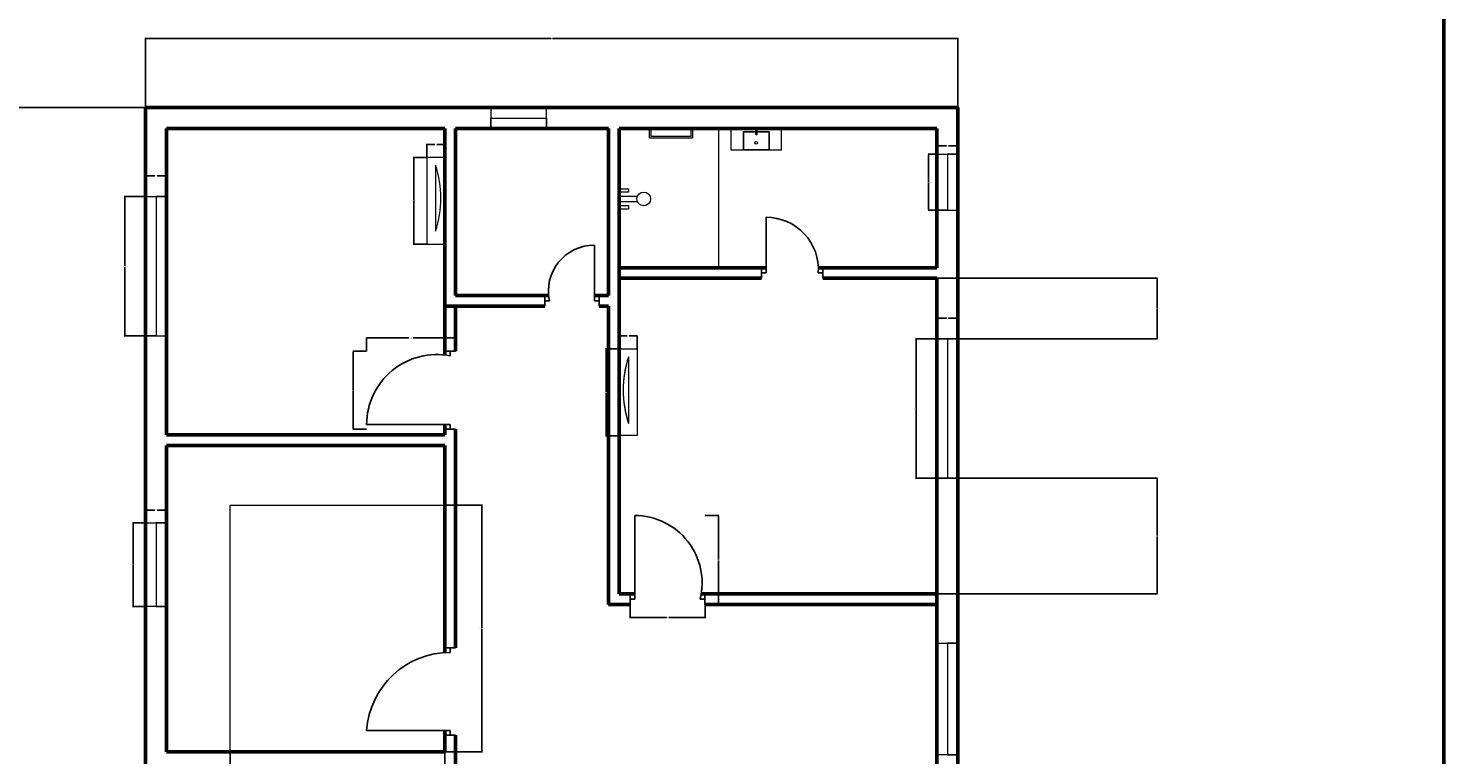
# Model space of a CAD drawing. Units: inches. Extents: x 2268 to 3372, y 1709 to 2892.
# Tile 5 of 6: x 2762 to 3372, y 2184 to 2497. Entities that reach past the tile are written whole.
import ezdxf

# ---------------------------------------------------------------- set-up
doc = ezdxf.new("R2010")
doc.units = ezdxf.units.IN
for name, color, linetype, lineweight in [('A-ANNO-DIMS', 2, 'Continuous', 18), ('A-ANNO-TTLB', 7, 'Continuous', 50), ('A-DOOR', 3, 'Continuous', 25), ('A-FLOR-FIXT', 9, 'Continuous', 18), ('A-FURN', 8, 'Continuous', 18), ('A-GLAZ', 4, 'Continuous', 18), ('A-WALL', 7, 'Continuous', 50)]:
    doc.layers.add(name, color=color, linetype=linetype, lineweight=lineweight)
doc.styles.get("Standard").update_dxf_attribs({"font": 'arial.ttf'})
doc.dimstyles.get("Standard").update_dxf_attribs({"dimtxt": 0.18, "dimasz": 0.18, "dimexe": 0.18, "dimexo": 0.0625, "dimgap": 0.09, "dimtad": 0, "dimtih": 1, "dimtoh": 1, "dimdec": 4, "dimzin": 0, "dimdsep": 46, "dimtxsty": 'Standard', "dimcen": 0.09, "dimadec": 0, "dimazin": 0, "dimtfac": 1, "dimtdec": 4, "dimtofl": 0, "dimtmove": 0, "dimatfit": 3, "dimfxl": 1, "dimtolj": 1, "dimtzin": 0, "dimarcsym": 0})

# ---------------------------------------------------------------- blocks, each defined once
blk = doc.blocks.new('DOOR-BEDROOM-E')
for p, q in [((2, 2.25), (2, 38.25)), ((0, 4.5), (0, 0)), ((0, 0), (0, 2.25)), ((0, 2.25), (2, 2.25)), ((32.14, 2.25), (30.14, 2.25)), ((32.14, 4.5), (32.14, 0)), ((32.14, 0), (32.14, 2.25))]:
    blk.add_line(p, q)
blk.add_arc((2, 9.25), 29, 346.03043, 90)
blk = doc.blocks.new('DOOR-BATH-W')
for p, q in [((21.4, 2.25), (21.4, 26.25)), ((0, 4.5), (0, 0)), ((0, 0), (0, 2.25)), ((0, 2.25), (2, 2.25)), ((23.4, 2.25), (21.4, 2.25)), ((23.4, 4.5), (23.4, 0)), ((23.4, 0), (23.4, 2.25))]:
    blk.add_line(p, q)
blk.add_arc((21.4, 6.41), 19.84, 90, 192.08962)
blk = doc.blocks.new('DOOR-BEDROOM-NW')
for p, q in [((33.75, 33.55), (38.25, 33.55)), ((38.25, 33.55), (36, 33.55)), ((36, 33.55), (36, 31.55)), ((36, 2), (0, 2)), ((33.75, 0), (38.25, 0)), ((36, 0), (36, 2)), ((38.25, 0), (36, 0))]:
    blk.add_line(p, q)
blk.add_arc((30.13, 2), 30.13, 78.75953, 180)
blk = doc.blocks.new('DOOR-BATH-E')
for p, q in [((2, 2.25), (2, 26.25)), ((0, 4.5), (0, 0)), ((0, 0), (0, 2.25)), ((0, 2.25), (2, 2.25)), ((26.44, 2.25), (24.44, 2.25)), ((26.44, 4.5), (26.44, 0)), ((26.44, 0), (26.44, 2.25))]:
    blk.add_line(p, q)
blk.add_arc((2, 3.76), 22.49, 356.14758, 90)
blk = doc.blocks.new('DOOR-KITCHEN')
for p, q in [((33.75, 37.66), (38.25, 37.66)), ((38.25, 37.66), (36, 37.66)), ((36, 37.66), (36, 35.66)), ((36, 2), (0, 2)), ((36, 0), (36, 2)), ((33.75, 0), (38.25, 0)), ((38.25, 0), (36, 0))]:
    blk.add_line(p, q)
blk.add_arc((36, -0.42), 36.08, 90, 176.1494)
blk = doc.blocks.new('WIN-60-SPLIT')
for p, q in [((0, 60), (9, 60)), ((9, 60), (4.5, 60)), ((4.5, 60), (4.5, 12)), ((4.5, 12), (4.5, 0)), ((4.5, 0), (0, 0)), ((0, 0), (9, 0))]:
    blk.add_line(p, q)
blk = doc.blocks.new('WIN-36')
for p, q in [((0, 36), (9, 36)), ((9, 36), (4.5, 36)), ((4.5, 36), (4.5, 0)), ((9, 0), (0, 0)), ((4.5, 0), (9, 0))]:
    blk.add_line(p, q)
blk = doc.blocks.new('WIN-24-TRANSVERSE')
for p, q in [((0, 9), (0, 0)), ((24, 0), (24, 9)), ((0, 0), (0, 4.5)), ((0, 4.5), (24, 4.5)), ((24, 4.5), (24, 0))]:
    blk.add_line(p, q)
blk = doc.blocks.new('WIN-24-LONGITUDINAL')
for p, q in [((0, 24), (9, 24)), ((9, 24), (4.5, 24)), ((4.5, 24), (4.5, 0)), ((4.5, 0), (0, 0)), ((0, 0), (9, 0))]:
    blk.add_line(p, q)
blk = doc.blocks.new('WIN-60-ALTERNATE')
for p, q in [((0, 60), (9, 60)), ((9, 60), (4.5, 60)), ((4.5, 60), (4.5, 0)), ((4.5, 0), (0, 0)), ((0, 0), (9, 0))]:
    blk.add_line(p, q)
blk = doc.blocks.new('WIN-48-ALTERNATE')
for p, q in [((0, 48), (9, 48)), ((9, 48), (4.5, 48)), ((4.5, 48), (4.5, 0)), ((9, 0), (0, 0)), ((4.5, 0), (9, 0))]:
    blk.add_line(p, q)
blk = doc.blocks.new('COUNTER-KITCHEN-L')
for p, q in [((0, 0), (0, 106.22)), ((0, 106.22), (92.56, 106.22))]:
    blk.add_line(p, q)
blk = doc.blocks.new('LAVATORY-VANITY')
for points in [[(0, 9.35), (21.53, 9.35), (21.53, 0), (0, 0)], [(10.67, 8.74), (11.01, 8.74), (11.01, 6.59), (10.67, 6.59)]]:
    blk.add_lwpolyline(points, close=True)
for points in [[(11.01, 8.1), (16.38, 8.1), (16.38, 0), (5.34, 0), (5.34, 8.1), (10.67, 8.1)], [(11.01, 7.98), (16.25, 7.98), (16.25, 0.14), (5.47, 0.14), (5.47, 7.98), (10.67, 7.98)]]:
    blk.add_lwpolyline(points)
blk.add_circle((10.78, 3.14), 0.562)
blk = doc.blocks.new('SHOWER-FITTING')
for points in [[(0, 8.74), (4.04, 8.74), (4.04, 7.26), (0, 7.26)], [(0, 1.48), (4.04, 1.48), (4.04, 0), (0, 0)]]:
    blk.add_lwpolyline(points, close=True)
blk.add_lwpolyline([(7.94, 3.17), (0, 3.17), (0, 5.6), (7.94, 5.6)])
blk.add_circle((10.64, 4.38), 2.96)
blk = doc.blocks.new('SHOWER-SHELF')
for points in [[(0, 4.16), (18.51, 4.16), (18.51, 0), (0, 0)], [(0.76, 4.16), (17.78, 4.16), (17.78, 0.69), (0.76, 0.69)]]:
    blk.add_lwpolyline(points, close=True)
blk = doc.blocks.new('BEDROOM-WALL-UNIT')
blk.add_line((3.85, 34.02), (3.85, 5.6))
blk.add_lwpolyline([(7.87, 37.37), (0, 37.37), (0, 0), (7.87, 0)], close=True)
blk.add_arc((-39.98, 19.81), 46.08, 342.03746, 17.96254)
blk = doc.blocks.new('BEDROOM-WALL-UNIT-E')
for p, q in [((4.02, 34.02), (4.02, 5.6)), ((4.02, 33.67), (4.02, 5.25))]:
    blk.add_line(p, q)
blk.add_lwpolyline([(0, 37.37), (7.87, 37.37), (7.87, 0), (0, 0)], close=True)
for centre in [(47.85, 19.81), (47.85, 19.46)]:
    blk.add_arc(centre, 46.08, 162.03746, 197.96254)
blk = doc.blocks.new('*D32')
at = {"layer": 'A-ANNO-DIMS', "color": 0, "lineweight": -2, "transparency": 16777216}
for p, q in [((3054.14, 2287.43), (3060, 2287.43)), ((3059.82, 2287.25), (3059.82, 2268.48)), ((3059.82, 2249.36), (3059.82, 2268.12)), ((3054.14, 2249.18), (3060, 2249.18))]:
    blk.add_line(p, q, dxfattribs=at)
at = {"layer": 'A-ANNO-DIMS', "color": 0, "transparency": 16777216}
for points in [[(3059.79, 2287.25), (3059.85, 2287.25), (3059.82, 2287.43)], [(3059.79, 2249.36), (3059.85, 2249.36), (3059.82, 2249.18)]]:
    blk.add_solid(points, dxfattribs=at)
at = {"layer": 'Defpoints', "color": 0, "transparency": 16777216}
for p in [(3054.08, 2287.43), (3059.82, 2287.43), (3054.08, 2249.18)]:
    blk.add_point(p, dxfattribs=at)
at = {"layer": 'A-ANNO-DIMS', "color": 0, "transparency": 16777216, "insert": (3059.82, 2268.3), "char_height": 0.18, "attachment_point": 5}
blk.add_mtext('\\A1;DOOR 38 TYP.', dxfattribs=at)
blk = doc.blocks.new('*D33')
at = {"layer": 'A-ANNO-DIMS', "color": 0, "lineweight": -2, "transparency": 16777216}
for p, q in [((3021.79, 2249.11), (3021.79, 2243.26)), ((3054.08, 2249.11), (3054.08, 2243.26)), ((3021.97, 2243.44), (3037.41, 2243.44)), ((3053.9, 2243.44), (3038.46, 2243.44))]:
    blk.add_line(p, q, dxfattribs=at)
at = {"layer": 'A-ANNO-DIMS', "color": 0, "transparency": 16777216}
for points in [[(3021.97, 2243.47), (3021.97, 2243.41), (3021.79, 2243.44)], [(3053.9, 2243.47), (3053.9, 2243.41), (3054.08, 2243.44)]]:
    blk.add_solid(points, dxfattribs=at)
at = {"layer": 'Defpoints', "color": 0, "transparency": 16777216}
for p in [(3021.79, 2249.18), (3054.08, 2249.18), (3054.08, 2243.44)]:
    blk.add_point(p, dxfattribs=at)
at = {"layer": 'A-ANNO-DIMS', "color": 0, "transparency": 16777216, "insert": (3037.93, 2243.44), "char_height": 0.18, "attachment_point": 5}
blk.add_mtext('\\A1;32 TYP.', dxfattribs=at)
blk = doc.blocks.new('*D36')
at = {"layer": 'A-ANNO-DIMS', "color": 0, "lineweight": -2, "transparency": 16777216}
for p, q in [((2908.25, 2358.25), (2908.25, 2364.1)), ((2908.43, 2363.92), (2926.44, 2363.92)), ((2946.32, 2363.92), (2928.31, 2363.92)), ((2946.5, 2358.25), (2946.5, 2364.1))]:
    blk.add_line(p, q, dxfattribs=at)
at = {"layer": 'A-ANNO-DIMS', "color": 0, "transparency": 16777216}
for points in [[(2908.43, 2363.95), (2908.43, 2363.89), (2908.25, 2363.92)], [(2946.32, 2363.95), (2946.32, 2363.89), (2946.5, 2363.92)]]:
    blk.add_solid(points, dxfattribs=at)
at = {"layer": 'Defpoints', "color": 0, "transparency": 16777216}
for p in [(2946.5, 2363.92), (2908.25, 2358.19), (2946.5, 2358.19)]:
    blk.add_point(p, dxfattribs=at)
at = {"layer": 'A-ANNO-DIMS', "color": 0, "transparency": 16777216, "insert": (2927.38, 2363.92), "char_height": 0.18, "attachment_point": 5}
blk.add_mtext('\\A1;DOOR 38 TYP.', dxfattribs=at)
blk = doc.blocks.new('*D37')
at = {"layer": 'A-ANNO-DIMS', "color": 0, "lineweight": -2, "transparency": 16777216}
for p, q in [((2908.19, 2358.19), (2902.33, 2358.19)), ((2902.51, 2358.01), (2902.51, 2341.59)), ((2902.51, 2324.82), (2902.51, 2341.23)), ((2908.19, 2324.64), (2902.33, 2324.64))]:
    blk.add_line(p, q, dxfattribs=at)
at = {"layer": 'A-ANNO-DIMS', "color": 0, "transparency": 16777216}
for points in [[(2902.48, 2358.01), (2902.54, 2358.01), (2902.51, 2358.19)], [(2902.48, 2324.82), (2902.54, 2324.82), (2902.51, 2324.64)]]:
    blk.add_solid(points, dxfattribs=at)
at = {"layer": 'Defpoints', "color": 0, "transparency": 16777216}
for p in [(2902.51, 2358.19), (2908.25, 2358.19), (2908.25, 2324.64)]:
    blk.add_point(p, dxfattribs=at)
at = {"layer": 'A-ANNO-DIMS', "color": 0, "transparency": 16777216, "insert": (2902.51, 2341.41), "char_height": 0.18, "attachment_point": 5}
blk.add_mtext('\\A1;34 TYP.', dxfattribs=at)
blk = doc.blocks.new('*D44')
at = {"layer": 'A-ANNO-DIMS', "color": 0, "lineweight": -2, "transparency": 16777216}
for p, q in [((2812.94, 2424.81), (2803.82, 2424.81)), ((2804, 2424.63), (2804, 2395)), ((2804, 2364.99), (2804, 2394.63)), ((2812.94, 2364.81), (2803.82, 2364.81))]:
    blk.add_line(p, q, dxfattribs=at)
at = {"layer": 'A-ANNO-DIMS', "color": 0, "transparency": 16777216}
for points in [[(2803.97, 2424.63), (2804.03, 2424.63), (2804, 2424.81)], [(2803.97, 2364.99), (2804.03, 2364.99), (2804, 2364.81)]]:
    blk.add_solid(points, dxfattribs=at)
at = {"layer": 'Defpoints', "color": 0, "transparency": 16777216}
for p in [(2804, 2424.81), (2813, 2424.81), (2813, 2364.81)]:
    blk.add_point(p, dxfattribs=at)
at = {"layer": 'A-ANNO-DIMS', "color": 0, "transparency": 16777216, "insert": (2804, 2394.81), "char_height": 0.18, "attachment_point": 5}
blk.add_mtext('\\A1;SPLIT WINDOW 60 TYP.', dxfattribs=at)
blk = doc.blocks.new('*D45')
at = {"layer": 'A-ANNO-DIMS', "color": 0, "lineweight": -2, "transparency": 16777216}
for p, q in [((2813, 2424.88), (2813, 2433.99)), ((2813.18, 2433.81), (2817.04, 2433.81)), ((2821.82, 2433.81), (2817.96, 2433.81)), ((2822, 2424.88), (2822, 2433.99))]:
    blk.add_line(p, q, dxfattribs=at)
at = {"layer": 'A-ANNO-DIMS', "color": 0, "transparency": 16777216}
for points in [[(2813.18, 2433.84), (2813.18, 2433.78), (2813, 2433.81)], [(2821.82, 2433.84), (2821.82, 2433.78), (2822, 2433.81)]]:
    blk.add_solid(points, dxfattribs=at)
at = {"layer": 'Defpoints', "color": 0, "transparency": 16777216}
for p in [(2822, 2433.81), (2813, 2424.81), (2822, 2424.81)]:
    blk.add_point(p, dxfattribs=at)
at = {"layer": 'A-ANNO-DIMS', "color": 0, "transparency": 16777216, "insert": (2817.5, 2433.81), "char_height": 0.18, "attachment_point": 5}
blk.add_mtext('\\A1;9 TYP.', dxfattribs=at)
blk = doc.blocks.new('*D46')
at = {"layer": 'A-ANNO-DIMS', "color": 0, "lineweight": -2, "transparency": 16777216}
for p, q in [((2812.94, 2284.31), (2807.42, 2284.31)), ((2807.6, 2284.13), (2807.6, 2266.49)), ((2807.6, 2248.49), (2807.6, 2266.13)), ((2812.94, 2248.31), (2807.42, 2248.31))]:
    blk.add_line(p, q, dxfattribs=at)
at = {"layer": 'A-ANNO-DIMS', "color": 0, "transparency": 16777216}
for points in [[(2807.57, 2284.13), (2807.63, 2284.13), (2807.6, 2284.31)], [(2807.57, 2248.49), (2807.63, 2248.49), (2807.6, 2248.31)]]:
    blk.add_solid(points, dxfattribs=at)
at = {"layer": 'Defpoints', "color": 0, "transparency": 16777216}
for p in [(2807.6, 2284.31), (2813, 2284.31), (2813, 2248.31)]:
    blk.add_point(p, dxfattribs=at)
at = {"layer": 'A-ANNO-DIMS', "color": 0, "transparency": 16777216, "insert": (2807.6, 2266.31), "char_height": 0.18, "attachment_point": 5}
blk.add_mtext('\\A1;WINDOW 36 TYP.', dxfattribs=at)
blk = doc.blocks.new('*D47')
at = {"layer": 'A-ANNO-DIMS', "color": 0, "lineweight": -2, "transparency": 16777216}
for p, q in [((2813, 2284.37), (2813, 2289.89)), ((2813.18, 2289.71), (2817.04, 2289.71)), ((2821.82, 2289.71), (2817.96, 2289.71)), ((2822, 2284.37), (2822, 2289.89))]:
    blk.add_line(p, q, dxfattribs=at)
at = {"layer": 'A-ANNO-DIMS', "color": 0, "transparency": 16777216}
for points in [[(2813.18, 2289.74), (2813.18, 2289.68), (2813, 2289.71)], [(2821.82, 2289.74), (2821.82, 2289.68), (2822, 2289.71)]]:
    blk.add_solid(points, dxfattribs=at)
at = {"layer": 'Defpoints', "color": 0, "transparency": 16777216}
for p in [(2822, 2289.71), (2813, 2284.31), (2822, 2284.31)]:
    blk.add_point(p, dxfattribs=at)
at = {"layer": 'A-ANNO-DIMS', "color": 0, "transparency": 16777216, "insert": (2817.5, 2289.71), "char_height": 0.18, "attachment_point": 5}
blk.add_mtext('\\A1;9 TYP.', dxfattribs=at)
blk = doc.blocks.new('*D50')
at = {"layer": 'A-ANNO-DIMS', "color": 0, "lineweight": -2, "transparency": 16777216}
for p, q in [((3153.94, 2443.05), (3150.22, 2443.05)), ((3150.4, 2442.87), (3150.4, 2431.24)), ((3150.4, 2419.23), (3150.4, 2430.87)), ((3153.94, 2419.05), (3150.22, 2419.05))]:
    blk.add_line(p, q, dxfattribs=at)
at = {"layer": 'A-ANNO-DIMS', "color": 0, "transparency": 16777216}
for points in [[(3150.37, 2442.87), (3150.43, 2442.87), (3150.4, 2443.05)], [(3150.37, 2419.23), (3150.43, 2419.23), (3150.4, 2419.05)]]:
    blk.add_solid(points, dxfattribs=at)
at = {"layer": 'Defpoints', "color": 0, "transparency": 16777216}
for p in [(3150.4, 2443.05), (3154, 2443.05), (3154, 2419.05)]:
    blk.add_point(p, dxfattribs=at)
at = {"layer": 'A-ANNO-DIMS', "color": 0, "transparency": 16777216, "insert": (3150.4, 2431.05), "char_height": 0.18, "attachment_point": 5}
blk.add_mtext('\\A1;WINDOW 24 TYP.', dxfattribs=at)
blk = doc.blocks.new('*D51')
at = {"layer": 'A-ANNO-DIMS', "color": 0, "lineweight": -2, "transparency": 16777216}
for p, q in [((3154, 2443.12), (3154, 2446.83)), ((3154.18, 2446.65), (3158.04, 2446.65)), ((3162.82, 2446.65), (3158.96, 2446.65)), ((3163, 2443.12), (3163, 2446.83))]:
    blk.add_line(p, q, dxfattribs=at)
at = {"layer": 'A-ANNO-DIMS', "color": 0, "transparency": 16777216}
for points in [[(3154.18, 2446.68), (3154.18, 2446.62), (3154, 2446.65)], [(3162.82, 2446.68), (3162.82, 2446.62), (3163, 2446.65)]]:
    blk.add_solid(points, dxfattribs=at)
at = {"layer": 'Defpoints', "color": 0, "transparency": 16777216}
for p in [(3163, 2446.65), (3154, 2443.05), (3163, 2443.05)]:
    blk.add_point(p, dxfattribs=at)
at = {"layer": 'A-ANNO-DIMS', "color": 0, "transparency": 16777216, "insert": (3158.5, 2446.65), "char_height": 0.18, "attachment_point": 5}
blk.add_mtext('\\A1;9 TYP.', dxfattribs=at)
blk = doc.blocks.new('*D52')
at = {"layer": 'A-ANNO-DIMS', "color": 0, "lineweight": -2, "transparency": 16777216}
for p, q in [((3153.94, 2363.53), (3144.82, 2363.53)), ((3145, 2363.35), (3145, 2333.71)), ((3145, 2303.71), (3145, 2333.35)), ((3153.94, 2303.53), (3144.82, 2303.53))]:
    blk.add_line(p, q, dxfattribs=at)
at = {"layer": 'A-ANNO-DIMS', "color": 0, "transparency": 16777216}
for points in [[(3144.97, 2363.35), (3145.03, 2363.35), (3145, 2363.53)], [(3144.97, 2303.71), (3145.03, 2303.71), (3145, 2303.53)]]:
    blk.add_solid(points, dxfattribs=at)
at = {"layer": 'Defpoints', "color": 0, "transparency": 16777216}
for p in [(3145, 2363.53), (3154, 2363.53), (3154, 2303.53)]:
    blk.add_point(p, dxfattribs=at)
at = {"layer": 'A-ANNO-DIMS', "color": 0, "transparency": 16777216, "insert": (3145, 2333.53), "char_height": 0.18, "attachment_point": 5}
blk.add_mtext('\\A1;WINDOW 60 TYP.', dxfattribs=at)
blk = doc.blocks.new('*D53')
at = {"layer": 'A-ANNO-DIMS', "color": 0, "lineweight": -2, "transparency": 16777216}
for p, q in [((3154, 2363.59), (3154, 2372.71)), ((3154.18, 2372.53), (3158.04, 2372.53)), ((3162.82, 2372.53), (3158.96, 2372.53)), ((3163, 2363.59), (3163, 2372.71))]:
    blk.add_line(p, q, dxfattribs=at)
at = {"layer": 'A-ANNO-DIMS', "color": 0, "transparency": 16777216}
for points in [[(3154.18, 2372.56), (3154.18, 2372.5), (3154, 2372.53)], [(3162.82, 2372.56), (3162.82, 2372.5), (3163, 2372.53)]]:
    blk.add_solid(points, dxfattribs=at)
at = {"layer": 'Defpoints', "color": 0, "transparency": 16777216}
for p in [(3163, 2372.53), (3154, 2363.53), (3163, 2363.53)]:
    blk.add_point(p, dxfattribs=at)
at = {"layer": 'A-ANNO-DIMS', "color": 0, "transparency": 16777216, "insert": (3158.5, 2372.53), "char_height": 0.18, "attachment_point": 5}
blk.add_mtext('\\A1;9 TYP.', dxfattribs=at)
blk = doc.blocks.new('*D58')
at = {"layer": 'A-ANNO-DIMS', "color": 0, "lineweight": -2, "transparency": 16777216}
for p, q in [((2942.06, 2291.9), (2958.11, 2291.9)), ((2957.93, 2291.72), (2957.93, 2238.97)), ((2957.93, 2185.86), (2957.93, 2238.6)), ((2942.06, 2185.68), (2958.11, 2185.68))]:
    blk.add_line(p, q, dxfattribs=at)
at = {"layer": 'A-ANNO-DIMS', "color": 0, "transparency": 16777216}
for points in [[(2957.9, 2291.72), (2957.96, 2291.72), (2957.93, 2291.9)], [(2957.9, 2185.86), (2957.96, 2185.86), (2957.93, 2185.68)]]:
    blk.add_solid(points, dxfattribs=at)
at = {"layer": 'Defpoints', "color": 0, "transparency": 16777216}
for p in [(2942, 2291.9), (2957.93, 2291.9), (2942, 2185.68)]:
    blk.add_point(p, dxfattribs=at)
at = {"layer": 'A-ANNO-DIMS', "color": 0, "transparency": 16777216, "insert": (2957.93, 2238.79), "char_height": 0.18, "attachment_point": 5}
blk.add_mtext('\\A1;COUNTER 106 TYP.', dxfattribs=at)
blk = doc.blocks.new('*D59')
at = {"layer": 'A-ANNO-DIMS', "color": 0, "lineweight": -2, "transparency": 16777216}
for p, q in [((2849.44, 2185.61), (2849.44, 2169.56)), ((2942, 2185.61), (2942, 2169.56)), ((2849.62, 2169.74), (2895.19, 2169.74)), ((2941.82, 2169.74), (2896.25, 2169.74))]:
    blk.add_line(p, q, dxfattribs=at)
at = {"layer": 'A-ANNO-DIMS', "color": 0, "transparency": 16777216}
for points in [[(2849.62, 2169.77), (2849.62, 2169.71), (2849.44, 2169.74)], [(2941.82, 2169.77), (2941.82, 2169.71), (2942, 2169.74)]]:
    blk.add_solid(points, dxfattribs=at)
at = {"layer": 'Defpoints', "color": 0, "transparency": 16777216}
for p in [(2849.44, 2185.68), (2942, 2185.68), (2942, 2169.74)]:
    blk.add_point(p, dxfattribs=at)
at = {"layer": 'A-ANNO-DIMS', "color": 0, "transparency": 16777216, "insert": (2895.72, 2169.74), "char_height": 0.18, "attachment_point": 5}
blk.add_mtext('\\A1;93 TYP.', dxfattribs=at)
blk = doc.blocks.new('*D66')
at = {"layer": 'A-ANNO-DIMS', "color": 0, "lineweight": -2, "transparency": 16777216}
for p, q in [((2934.07, 2441.71), (2928.35, 2441.71)), ((2928.53, 2441.53), (2928.53, 2423.21)), ((2928.53, 2404.53), (2928.53, 2422.85)), ((2934.07, 2404.35), (2928.35, 2404.35))]:
    blk.add_line(p, q, dxfattribs=at)
at = {"layer": 'A-ANNO-DIMS', "color": 0, "transparency": 16777216}
for points in [[(2928.5, 2441.53), (2928.56, 2441.53), (2928.53, 2441.71)], [(2928.5, 2404.53), (2928.56, 2404.53), (2928.53, 2404.35)]]:
    blk.add_solid(points, dxfattribs=at)
at = {"layer": 'Defpoints', "color": 0, "transparency": 16777216}
for p in [(2928.53, 2441.71), (2934.14, 2441.71), (2934.14, 2404.35)]:
    blk.add_point(p, dxfattribs=at)
at = {"layer": 'A-ANNO-DIMS', "color": 0, "transparency": 16777216, "insert": (2928.53, 2423.03), "char_height": 0.18, "attachment_point": 5}
blk.add_mtext('\\A1;WALL UNIT 37 TYP.', dxfattribs=at)
blk = doc.blocks.new('*D67')
at = {"layer": 'A-ANNO-DIMS', "color": 0, "lineweight": -2, "transparency": 16777216}
for p, q in [((2934.14, 2441.78), (2934.14, 2447.5)), ((2934.32, 2447.32), (2937.61, 2447.32)), ((2941.82, 2447.32), (2938.53, 2447.32)), ((2942, 2441.78), (2942, 2447.5))]:
    blk.add_line(p, q, dxfattribs=at)
at = {"layer": 'A-ANNO-DIMS', "color": 0, "transparency": 16777216}
for points in [[(2934.32, 2447.35), (2934.32, 2447.29), (2934.14, 2447.32)], [(2941.82, 2447.35), (2941.82, 2447.29), (2942, 2447.32)]]:
    blk.add_solid(points, dxfattribs=at)
at = {"layer": 'Defpoints', "color": 0, "transparency": 16777216}
for p in [(2942, 2447.32), (2934.14, 2441.71), (2942, 2441.71)]:
    blk.add_point(p, dxfattribs=at)
at = {"layer": 'A-ANNO-DIMS', "color": 0, "transparency": 16777216, "insert": (2938.07, 2447.32), "char_height": 0.18, "attachment_point": 5}
blk.add_mtext('\\A1;8 TYP.', dxfattribs=at)
blk = doc.blocks.new('*D68')
at = {"layer": 'A-ANNO-DIMS', "color": 0, "lineweight": -2, "transparency": 16777216}
for p, q in [((3016.94, 2359.21), (3011.22, 2359.21)), ((3011.4, 2359.03), (3011.4, 2340.71)), ((3011.4, 2322.02), (3011.4, 2340.34)), ((3016.94, 2321.84), (3011.22, 2321.84))]:
    blk.add_line(p, q, dxfattribs=at)
at = {"layer": 'A-ANNO-DIMS', "color": 0, "transparency": 16777216}
for points in [[(3011.37, 2359.03), (3011.43, 2359.03), (3011.4, 2359.21)], [(3011.37, 2322.02), (3011.43, 2322.02), (3011.4, 2321.84)]]:
    blk.add_solid(points, dxfattribs=at)
at = {"layer": 'Defpoints', "color": 0, "transparency": 16777216}
for p in [(3011.4, 2359.21), (3017, 2359.21), (3017, 2321.84)]:
    blk.add_point(p, dxfattribs=at)
at = {"layer": 'A-ANNO-DIMS', "color": 0, "transparency": 16777216, "insert": (3011.4, 2340.53), "char_height": 0.18, "attachment_point": 5}
blk.add_mtext('\\A1;WALL UNIT 37 TYP.', dxfattribs=at)
blk = doc.blocks.new('*D69')
at = {"layer": 'A-ANNO-DIMS', "color": 0, "lineweight": -2, "transparency": 16777216}
for p, q in [((3017, 2359.27), (3017, 2365)), ((3017.18, 2364.82), (3020.48, 2364.82)), ((3024.69, 2364.82), (3021.39, 2364.82)), ((3024.87, 2359.27), (3024.87, 2365))]:
    blk.add_line(p, q, dxfattribs=at)
at = {"layer": 'A-ANNO-DIMS', "color": 0, "transparency": 16777216}
for points in [[(3017.18, 2364.85), (3017.18, 2364.79), (3017, 2364.82)], [(3024.69, 2364.85), (3024.69, 2364.79), (3024.87, 2364.82)]]:
    blk.add_solid(points, dxfattribs=at)
at = {"layer": 'Defpoints', "color": 0, "transparency": 16777216}
for p in [(3024.87, 2364.82), (3017, 2359.21), (3024.87, 2359.21)]:
    blk.add_point(p, dxfattribs=at)
at = {"layer": 'A-ANNO-DIMS', "color": 0, "transparency": 16777216, "insert": (3020.93, 2364.82), "char_height": 0.18, "attachment_point": 5}
blk.add_mtext('\\A1;8 TYP.', dxfattribs=at)
blk = doc.blocks.new('*D92')
at = {"layer": 'A-ANNO-DIMS', "color": 0, "lineweight": -2, "transparency": 16777216}
for p, q in [((2813, 2463.24), (2813, 2493.16)), ((2813.18, 2492.98), (2987.71, 2492.98)), ((3162.82, 2492.98), (2988.29, 2492.98)), ((3163, 2463.24), (3163, 2493.16))]:
    blk.add_line(p, q, dxfattribs=at)
at = {"layer": 'A-ANNO-DIMS', "color": 0, "transparency": 16777216}
for points in [[(2813.18, 2493.01), (2813.18, 2492.95), (2813, 2492.98)], [(3162.82, 2493.01), (3162.82, 2492.95), (3163, 2492.98)]]:
    blk.add_solid(points, dxfattribs=at)
at = {"layer": 'Defpoints', "color": 0, "transparency": 16777216}
for p in [(3163, 2492.98), (2813, 2463.18), (3163, 2463.18)]:
    blk.add_point(p, dxfattribs=at)
at = {"layer": 'A-ANNO-DIMS', "color": 0, "transparency": 16777216, "insert": (2988, 2492.98), "char_height": 0.18, "attachment_point": 5}
blk.add_mtext('\\A1;350', dxfattribs=at)
blk = doc.blocks.new('*D93')
at = {"layer": 'A-ANNO-DIMS', "color": 0, "lineweight": -2, "transparency": 16777216}
for p, q in [((2812.94, 2463.18), (2743.52, 2463.18)), ((2743.7, 2463), (2743.7, 2170.36)), ((2743.7, 1877.36), (2743.7, 2169.99)), ((2812.94, 1877.18), (2743.52, 1877.18))]:
    blk.add_line(p, q, dxfattribs=at)
at = {"layer": 'A-ANNO-DIMS', "color": 0, "transparency": 16777216}
for points in [[(2743.67, 2463), (2743.73, 2463), (2743.7, 2463.18)], [(2743.67, 1877.36), (2743.73, 1877.36), (2743.7, 1877.18)]]:
    blk.add_solid(points, dxfattribs=at)
at = {"layer": 'Defpoints', "color": 0, "transparency": 16777216}
for p in [(2743.7, 2463.18), (2813, 2463.18), (2813, 1877.18)]:
    blk.add_point(p, dxfattribs=at)
at = {"layer": 'A-ANNO-DIMS', "color": 0, "transparency": 16777216, "insert": (2743.7, 2170.18), "char_height": 0.18, "attachment_point": 5}
blk.add_mtext('\\A1;586', dxfattribs=at)
blk = doc.blocks.new('*D96')
at = {"layer": 'A-ANNO-DIMS', "color": 0, "lineweight": -2, "transparency": 16777216}
for p, q in [((3154.06, 2303.53), (3249.09, 2303.53)), ((3248.91, 2303.35), (3248.91, 2278.79)), ((3248.91, 2253.86), (3248.91, 2278.42)), ((3154.06, 2253.68), (3249.09, 2253.68))]:
    blk.add_line(p, q, dxfattribs=at)
at = {"layer": 'A-ANNO-DIMS', "color": 0, "transparency": 16777216}
for points in [[(3248.88, 2303.35), (3248.94, 2303.35), (3248.91, 2303.53)], [(3248.88, 2253.86), (3248.94, 2253.86), (3248.91, 2253.68)]]:
    blk.add_solid(points, dxfattribs=at)
at = {"layer": 'Defpoints', "color": 0, "transparency": 16777216}
for p in [(3154, 2303.53), (3248.91, 2303.53), (3154, 2253.68)]:
    blk.add_point(p, dxfattribs=at)
at = {"layer": 'A-ANNO-DIMS', "color": 0, "transparency": 16777216, "insert": (3248.91, 2278.6), "char_height": 0.18, "attachment_point": 5}
blk.add_mtext('\\A1;49.86', dxfattribs=at)
blk = doc.blocks.new('*D97')
at = {"layer": 'A-ANNO-DIMS', "color": 0, "lineweight": -2, "transparency": 16777216}
for p, q in [((3154.06, 2389.68), (3249.09, 2389.68)), ((3248.91, 2389.5), (3248.91, 2376.79)), ((3248.91, 2363.71), (3248.91, 2376.42)), ((3154.06, 2363.53), (3249.09, 2363.53))]:
    blk.add_line(p, q, dxfattribs=at)
at = {"layer": 'A-ANNO-DIMS', "color": 0, "transparency": 16777216}
for points in [[(3248.88, 2389.5), (3248.94, 2389.5), (3248.91, 2389.68)], [(3248.88, 2363.71), (3248.94, 2363.71), (3248.91, 2363.53)]]:
    blk.add_solid(points, dxfattribs=at)
at = {"layer": 'Defpoints', "color": 0, "transparency": 16777216}
for p in [(3154, 2389.68), (3248.91, 2389.68), (3154, 2363.53)]:
    blk.add_point(p, dxfattribs=at)
at = {"layer": 'A-ANNO-DIMS', "color": 0, "transparency": 16777216, "insert": (3248.91, 2376.6), "char_height": 0.18, "attachment_point": 5}
blk.add_mtext('\\A1;26.145', dxfattribs=at)

msp = doc.modelspace()

# ---------------------------------------------------------------- linework, layer by layer
at = {"layer": 'A-ANNO-TTLB'}
msp.add_lwpolyline([(2268.3884, 2892.2471), (3372.3464, 2892.2471), (3372.3464, 1709.0755), (2268.3884, 1709.0755)], close=True, dxfattribs=at)
at = {"layer": 'A-FLOR-FIXT'}
msp.add_line((3059.8062, 2454.1756), (3059.8062, 2394.1756), dxfattribs=at)
at = {"layer": 'A-WALL'}
for p, q in [((2813.001, 2463.1756), (3163.001, 2463.1756)), ((2813.001, 2463.1756), (3163.001, 2463.1756)), ((2813.001, 2463.1756), (2813.001, 1877.1756)), ((3163.001, 2463.1756), (3163.001, 1877.1756)), ((2822.001, 2454.1756), (2942.001, 2454.1756)), ((2822.001, 2454.1756), (2822.001, 2322.1756)), ((2942.001, 2454.1756), (2942.001, 2356.5449)), ((2946.501, 2454.1756), (3012.501, 2454.1756)), ((2946.501, 2454.1756), (2946.501, 2382.1756)), ((3012.501, 2454.1756), (3012.501, 2382.1756)), ((3017.001, 2454.1756), (3154.001, 2454.1756)), ((3017.001, 2454.1756), (3017.001, 2253.6756)), ((3154.001, 2454.1756), (3154.001, 2394.1756)), ((3017.001, 2394.1756), (3080.4095, 2394.1756)), ((3102.8863, 2394.1756), (3154.001, 2394.1756)), ((3017.001, 2389.6756), (3078.4095, 2389.6756)), ((3104.8477, 2389.6756), (3154.001, 2389.6756)), ((3154.001, 2389.6756), (3154.001, 2049.1756)), ((2946.501, 2382.1756), (2986.6383, 2382.1756)), ((3006.3904, 2382.1756), (3012.501, 2382.1756)), ((2942.001, 2377.6756), (2984.9866, 2377.6756)), ((2946.501, 2377.6756), (2946.501, 2358.1856)), ((3008.3904, 2377.6756), (3012.501, 2377.6756)), ((3012.501, 2377.6756), (3012.501, 2249.1756)), ((2942.001, 2326.6361), (2942.001, 2322.1756)), ((2946.501, 2324.6361), (2946.501, 2230.4862)), ((2822.001, 2322.1756), (2942.001, 2322.1756)), ((2822.001, 2317.6756), (2942.001, 2317.6756)), ((2822.001, 2317.6756), (2822.001, 2185.6756)), ((2942.001, 2317.6756), (2942.001, 2228.4159)), ((3017.001, 2253.6756), (3023.7859, 2253.6756)), ((3052.3935, 2253.6756), (3154.001, 2253.6756)), ((3017.001, 2249.1756), (3012.501, 2249.1756)), ((3017.001, 2249.1756), (3021.7859, 2249.1756)), ((3053.9275, 2249.1756), (3154.001, 2249.1756)), ((2942.001, 2194.8278), (2942.001, 2185.6756)), ((2946.501, 2192.8278), (2946.501, 2174.6517)), ((2822.001, 2185.6756), (2942.001, 2185.6756))]:
    msp.add_line(p, q, dxfattribs=at)

# ---------------------------------------------------------------- block references
at = {"layer": 'A-DOOR'}
for name, p in [('DOOR-BATH-E', (3078.4097, 2389.676)), ('DOOR-BATH-W', (2984.9867, 2377.676)), ('DOOR-BEDROOM-NW', (2908.2507, 2324.636)), ('DOOR-BEDROOM-E', (3021.7857, 2249.176)), ('DOOR-KITCHEN', (2908.2507, 2192.828))]:
    msp.add_blockref(name, p, dxfattribs=at)
at = {"layer": 'A-FLOR-FIXT'}
for name, p in [('SHOWER-SHELF', (3030.1587, 2450.016)), ('LAVATORY-VANITY', (3065.3337, 2444.822)), ('SHOWER-FITTING', (3017.0007, 2419.462)), ('COUNTER-KITCHEN-L', (2849.4367, 2185.676))]:
    msp.add_blockref(name, p, dxfattribs=at)
at = {"layer": 'A-FURN'}
for name, p in [('BEDROOM-WALL-UNIT', (2934.1357, 2404.345)), ('BEDROOM-WALL-UNIT-E', (3017.0007, 2321.841))]:
    msp.add_blockref(name, p, dxfattribs=at)
at = {"layer": 'A-GLAZ'}
for name, p in [('WIN-24-TRANSVERSE', (2961.7967, 2454.176)), ('WIN-24-LONGITUDINAL', (3154.0007, 2419.053)), ('WIN-60-SPLIT', (2813.0007, 2364.813)), ('WIN-60-ALTERNATE', (3154.0007, 2303.531)), ('WIN-36', (2813.0007, 2248.308)), ('WIN-48-ALTERNATE', (3154.0007, 2184.405))]:
    msp.add_blockref(name, p, dxfattribs=at)

# ---------------------------------------------------------------- dimensions: what is measured, and where the dimension line sits
at = {"layer": 'A-ANNO-DIMS'}
dim = msp.add_linear_dim(base=(3163.001, 2492.9756), p1=(2813.001, 2463.1756), p2=(3163.001, 2463.1756), dimstyle='Standard', override={"dimdec": 0, "dimlfac": 1, "dimrnd": 0, "dimzin": 0, "dimdsep": 46, "dimlunit": 2}, dxfattribs=at)
dim.commit()
dim.dimension.update_dxf_attribs({"geometry": '*D92', "text_midpoint": (2988.001, 2492.9756)})
for base, p1, p2, override, picture, middle in [((2743.7041, 2463.1756), (2813.001, 1877.1756), (2813.001, 2463.1756), {"dimdec": 0, "dimlfac": 1, "dimrnd": 0, "dimzin": 0, "dimdsep": 46, "dimlunit": 2}, '*D93', (2743.7041, 2170.1756)), ((3248.91383, 2389.67559), (3154.001, 2363.53106), (3154.001, 2389.67559), {"dimdec": 3, "dimlfac": 1, "dimrnd": 0, "dimzin": 0, "dimdsep": 46, "dimlunit": 2}, '*D97', (3248.91383, 2376.60332)), ((3248.9138, 2303.5311), (3154.001, 2253.6756), (3154.001, 2303.5311), {"dimdec": 2, "dimlfac": 1, "dimrnd": 0, "dimzin": 0, "dimdsep": 46, "dimlunit": 2}, '*D96', (3248.9138, 2278.6033))]:
    dim = msp.add_linear_dim(base=base, p1=p1, p2=p2, angle=90, dimstyle='Standard', override=override, dxfattribs=at)
    dim.commit()
    dim.dimension.update_dxf_attribs({"geometry": picture, "text_midpoint": middle})
for base, p1, p2, text, picture, middle in [((2942.001, 2447.3193), (2934.1361, 2441.7139), (2942.001, 2441.7139), '<> TYP.', '*D67', (2938.0686, 2447.3193)), ((3163.001, 2446.6535), (3154.001, 2443.0535), (3163.001, 2443.0535), '<> TYP.', '*D51', (3158.501, 2446.6535)), ((2822.001, 2433.813), (2813.001, 2424.813), (2822.001, 2424.813), '<> TYP.', '*D45', (2817.501, 2433.813)), ((3163.001, 2372.5311), (3154.001, 2363.5311), (3163.001, 2363.5311), '<> TYP.', '*D53', (3158.501, 2372.5311)), ((2946.501, 2363.9231), (2908.251, 2358.1856), (2946.501, 2358.1856), 'DOOR <> TYP.', '*D36', (2927.376, 2363.9231)), ((3024.8659, 2364.8156), (3017.001, 2359.2102), (3024.8659, 2359.2102), '<> TYP.', '*D69', (3020.9334, 2364.8156)), ((2822.001, 2289.7084), (2813.001, 2284.3084), (2822.001, 2284.3084), '<> TYP.', '*D47', (2817.501, 2289.7084)), ((3054.0819, 2243.4381), (3021.7859, 2249.1756), (3054.0819, 2249.1756), '<> TYP.', '*D33', (3037.9339, 2243.4381)), ((2942.001, 2169.7422), (2849.4367, 2185.6756), (2942.001, 2185.6756), '<> TYP.', '*D59', (2895.7189, 2169.7422))]:
    dim = msp.add_linear_dim(base=base, p1=p1, p2=p2, text=text, dimstyle='Standard', override={"dimdec": 0, "dimlfac": 1, "dimrnd": 0, "dimzin": 0, "dimdsep": 46, "dimlunit": 2}, dxfattribs=at)
    dim.commit()
    dim.dimension.update_dxf_attribs({"geometry": picture, "text_midpoint": middle})
for base, p1, p2, text, picture, middle in [((2928.5308, 2441.7139), (2934.1361, 2404.345), (2934.1361, 2441.7139), 'WALL UNIT <> TYP.', '*D66', (2928.5308, 2423.0295)), ((3150.401, 2443.0535), (3154.001, 2419.0535), (3154.001, 2443.0535), 'WINDOW <> TYP.', '*D50', (3150.401, 2431.0535)), ((2804.001, 2424.813), (2813.001, 2364.813), (2813.001, 2424.813), 'SPLIT WINDOW <> TYP.', '*D44', (2804.001, 2394.813)), ((3145.001, 2363.5311), (3154.001, 2303.5311), (3154.001, 2363.5311), 'WINDOW <> TYP.', '*D52', (3145.001, 2333.5311)), ((2902.5135, 2358.1856), (2908.251, 2324.6361), (2908.251, 2358.1856), '<> TYP.', '*D37', (2902.5135, 2341.4109)), ((3011.3957, 2359.2102), (3017.001, 2321.8413), (3017.001, 2359.2102), 'WALL UNIT <> TYP.', '*D68', (3011.3957, 2340.5257)), ((2957.9344, 2291.8984), (2942.001, 2185.6756), (2942.001, 2291.8984), 'COUNTER <> TYP.', '*D58', (2957.9344, 2238.787)), ((3059.8194, 2287.4256), (3054.0819, 2249.1756), (3054.0819, 2287.4256), 'DOOR <> TYP.', '*D32', (3059.8194, 2268.3006)), ((2807.601, 2284.3084), (2813.001, 2248.3084), (2813.001, 2284.3084), 'WINDOW <> TYP.', '*D46', (2807.601, 2266.3084))]:
    dim = msp.add_linear_dim(base=base, p1=p1, p2=p2, angle=90, text=text, dimstyle='Standard', override={"dimdec": 0, "dimlfac": 1, "dimrnd": 0, "dimzin": 0, "dimdsep": 46, "dimlunit": 2}, dxfattribs=at)
    dim.commit()
    dim.dimension.update_dxf_attribs({"geometry": picture, "text_midpoint": middle})

doc.saveas('drawing.dxf')
